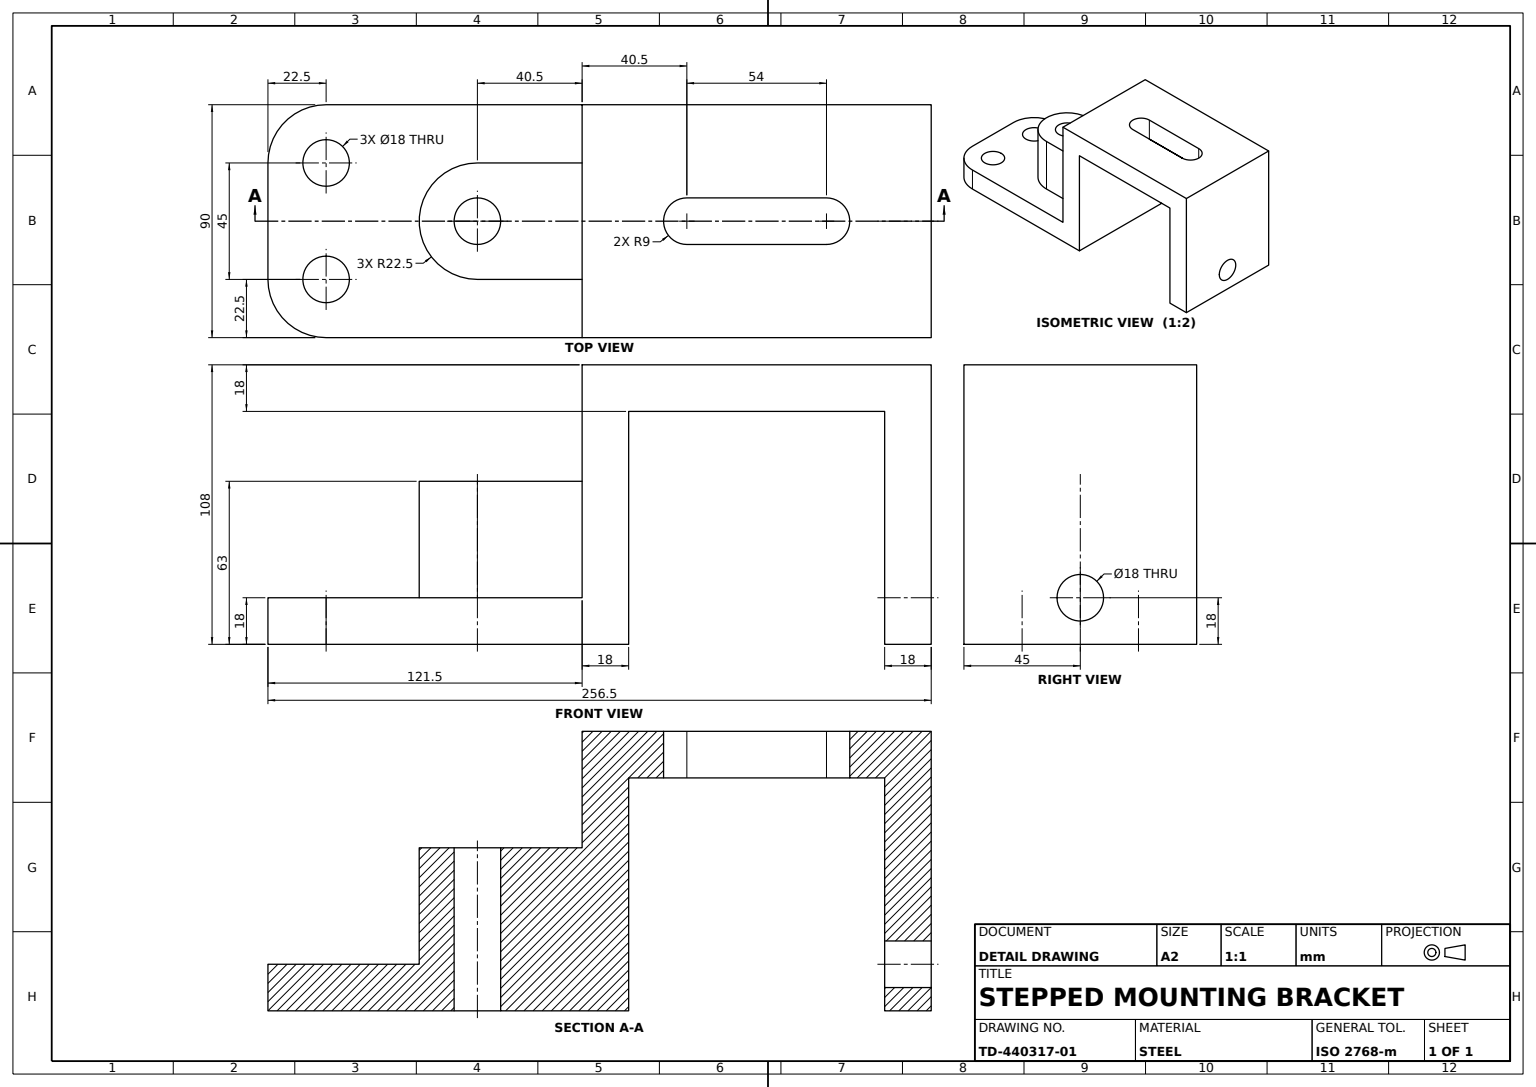
from build123d import *

# Parameters (mm, degrees)
BRACKET_BODY_DEPTH            = 45
TOP_SLOT_18X72_DEPTH          = 45
PIVOT_BOSS_DEPTH              = 45
PIVOT_BORE_SKETCH_R           = 9
PIVOT_BORE_18_DEPTH           = 72
FLANGE_CORNER_FILLETS_R22_5_R = 22.5
FLANGE_HOLES_SKETCH_R         = 9
FLANGE_HOLES_2X_18_DEPTH      = 72
SIDE_HOLE_SKETCH_R            = 9
SIDE_HOLE_18_DEPTH            = 72


with BuildPart() as part:
    # Bracket Profile Sketch → Bracket Body (new, symmetric)
    with BuildSketch(Plane.XY):
        Polygon((0, 0), (0, 18), (121.5, 18), (121.5, 108), (256.5, 108), (256.5, 0), (238.5, 0), (238.5, 90), (139.5, 90), (139.5, 0), align=None)
    extrude(amount=BRACKET_BODY_DEPTH, both=True)

    # Top Slot Sketch → Top Slot 18x72 (cut, symmetric)
    with BuildSketch(Plane(origin=(0, 108, 0), x_dir=(1, 0, 0), z_dir=(0, 1, 0))):
        with BuildLine():
            Line((162, 9), (216, 9))
            ThreePointArc((216, 9), (225, 0), (216, -9))
            Line((216, -9), (162, -9))
            ThreePointArc((162, -9), (153, 0), (162, 9))
        make_face()
    extrude(amount=TOP_SLOT_18X72_DEPTH, both=True, mode=Mode.SUBTRACT)

    # Pivot Boss Sketch → Pivot Boss (add)
    with BuildSketch(Plane(origin=(0, 18, 0), x_dir=(1, 0, 0), z_dir=(0, 1, 0))):
        with BuildLine():
            Line((81, 22.5), (121.5, 22.5))
            Line((121.5, 22.5), (121.5, -22.5))
            Line((121.5, -22.5), (81, -22.5))
            ThreePointArc((81, -22.5), (58.5, 0), (81, 22.5))
        make_face()
    extrude(amount=PIVOT_BOSS_DEPTH)

    # Pivot Bore Sketch → Pivot Bore Ø18 (cut)
    with BuildSketch(Plane(origin=(0, 63, 0), x_dir=(1, 0, 0), z_dir=(0, 1, 0))):
        with Locations(Location((81, 0, 0), (0, 0, 270))):
            Circle(PIVOT_BORE_SKETCH_R)
    extrude(amount=-PIVOT_BORE_18_DEPTH, mode=Mode.SUBTRACT)

    # Flange Corner Fillets R22.5
    flange_corner_fillets_r22_5_edges = [part.edges().sort_by_distance(p)[0] for p in [
        (0, 9, -45),
        (0, 9, 45),
    ]]
    fillet(flange_corner_fillets_r22_5_edges, radius=FLANGE_CORNER_FILLETS_R22_5_R)

    # Flange Holes Sketch → Flange Holes 2xØ18 (cut)
    with BuildSketch(Plane(origin=(0, 18, 0), x_dir=(1, 0, 0), z_dir=(0, 1, 0))):
        with Locations(Location((22.5, 22.5, 0), (0, 0, 270))):
            Circle(FLANGE_HOLES_SKETCH_R)
        with Locations(Location((22.5, -22.5, 0), (0, 0, 270))):
            Circle(FLANGE_HOLES_SKETCH_R)
    extrude(amount=-FLANGE_HOLES_2X_18_DEPTH, mode=Mode.SUBTRACT)

    # Side Hole Sketch → Side Hole Ø18 (cut)
    with BuildSketch(Plane(origin=(256.5, 0, 0), x_dir=(0, 0, -1), z_dir=(1, 0, 0))):
        with Locations((0, 18)):
            Circle(SIDE_HOLE_SKETCH_R)
    extrude(amount=-SIDE_HOLE_18_DEPTH, mode=Mode.SUBTRACT)


solid = part.part
